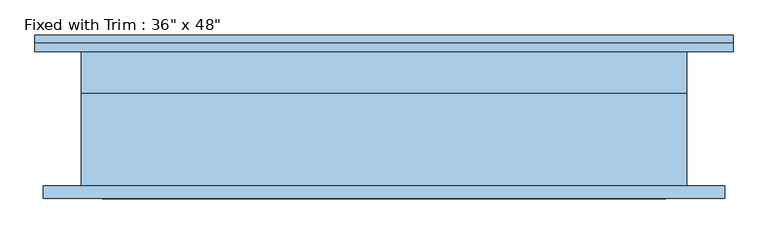
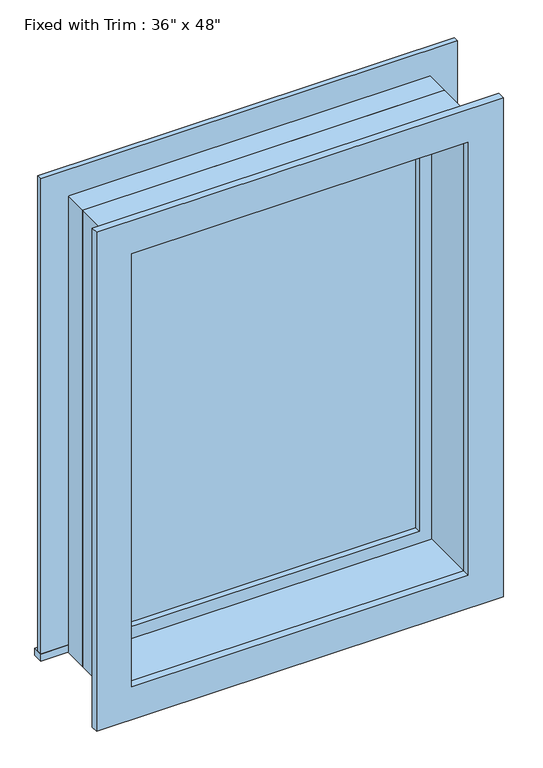
"""IFC4 building model written with IfcOpenShell, lengths in millimetres: window geometry."""

from ifc_helpers import new_model, si_unit, frame, origin, place, context, project, spatial, polyline, outline, extrude, source, transform, mapped, element, save


def window_bec2521a(model_context):
    return source(origin(), model_context, "Body", "SweptSolid", [
        extrude(outline(polyline([(-565.15, 127.0), (488.95, 127.0), (488.95, 101.6), (-565.15, 101.6), (-565.15, 127.0)])), frame((0.0, 0.0, 914.4), z_axis=(0.0, 0.0, 1.0), x_axis=(1.0, 0.0, 0.0)), (0.0, 0.0, 1.0), 19.05),
        extrude(outline(polyline([(2114.55, -476.25), (2114.55, 400.05), (933.45, 400.05), (933.45, 488.95), (2203.45, 488.95), (2203.45, -565.15), (933.45, -565.15), (933.45, -476.25), (2114.55, -476.25)])), frame((0.0, 101.6, 0.0), z_axis=(0.0, 1.0, 0.0), x_axis=(0.0, 0.0, 1.0)), (0.0, 0.0, 1.0), 12.7),
        extrude(outline(polyline([(2190.75, 476.25), (2190.75, -552.45), (857.25, -552.45), (857.25, 476.25), (2190.75, 476.25)]), holes=[polyline([(2101.85, 387.35), (946.15, 387.35), (946.15, -463.55), (2101.85, -463.55), (2101.85, 387.35)])]), frame((0.0, -120.65, 0.0), z_axis=(0.0, 1.0, 0.0), x_axis=(0.0, 0.0, 1.0)), (0.0, 0.0, 1.0), 19.05),
        extrude(outline(polyline([(355.6, 53.975), (-431.8, 53.975), (-431.8, 66.675), (355.6, 66.675), (355.6, 53.975)])), frame((0.0, 0.0, 977.9), z_axis=(0.0, 0.0, 1.0), x_axis=(1.0, 0.0, 0.0)), (0.0, 0.0, 1.0), 1092.2),
        extrude(outline(polyline([(2114.55, -476.25), (933.45, -476.25), (933.45, 400.05), (2114.55, 400.05), (2114.55, -476.25)]), holes=[polyline([(2070.1, -431.8), (2070.1, 355.6), (977.9, 355.6), (977.9, -431.8), (2070.1, -431.8)])]), frame((0.0, 38.1, 0.0), z_axis=(0.0, 1.0, 0.0), x_axis=(0.0, 0.0, 1.0)), (0.0, 0.0, 1.0), 44.45),
        extrude(outline(polyline([(2133.6, -495.3), (914.4, -495.3), (914.4, 419.1), (2133.6, 419.1), (2133.6, -495.3)]), holes=[polyline([(2101.85, -463.55), (2101.85, 387.35), (946.15, 387.35), (946.15, -463.55), (2101.85, -463.55)])]), frame((0.0, -101.6, 0.0), z_axis=(0.0, 1.0, 0.0), x_axis=(0.0, 0.0, 1.0)), (0.0, 0.0, 1.0), 139.7),
        extrude(outline(polyline([(2133.6, 419.1), (2133.6, -495.3), (914.4, -495.3), (914.4, 419.1), (2133.6, 419.1)]), holes=[polyline([(2114.55, 400.05), (933.45, 400.05), (933.45, -476.25), (2114.55, -476.25), (2114.55, 400.05)])]), frame((0.0, 38.1, 0.0), z_axis=(0.0, 1.0, 0.0), x_axis=(0.0, 0.0, 1.0)), (0.0, 0.0, 1.0), 63.5),
    ])


if __name__ == "__main__":
    model = new_model("IFC4")
    model_context = context("Model", 3, world=origin())
    ifc_project = project(units=[si_unit("LENGTHUNIT", "METRE", prefix="MILLI")], contexts=[model_context])
    site = spatial("IfcSite", under=ifc_project)
    building = spatial("IfcBuilding", under=site)
    placement = place(None, origin())
    window_shape = window_bec2521a(model_context)
    element("IfcWindow", 1, ObjectType="Fixed with Trim : 36\" x 48\"", at=placement, inside=building, context=model_context, shape_type="MappedRepresentation", body=[
        mapped(window_shape, transform((0.0, 0.0, 0.0), x_axis=(1.0, 0.0, 0.0), y_axis=(0.0, 1.0, 0.0), z_axis=(0.0, 0.0, 1.0))),
    ])
    save(model, "model.ifc")

# Revit data of these elements
# Type "Fixed with Trim : 36\" x 48\""
#   Type Mark = "13"
#   Construction Type Id = "GSP4R"
#   Assembly Code = "B2020100"
#   Analytic Construction = "1/8 in Pilkington single glazing"
#   Visual Light Transmittance = 0.9
#   Solar Heat Gain Coefficient = 0.78
#   Heat Transfer Coefficient (U) = 0.6496 BTU/(h·ft²·°F)
#   Height = 4' - 0"
#   Default Sill Height = 3' - 0"
#   Trim Projection - Ext. = 0' - 0 1/2"
#   Trim Projection - Int. = 0' - 0 3/4"
#   Trim Width - Exterior = 0' - 3 1/2"
#   Trim Width - Interior = 0' - 3 1/2"
#   Width = 3' - 0"
#   Window Inset = 0' - 0 3/4"
#   Define Thermal Properties by = 1
#   Glass Pane Material = Glass
#   Sash Material = Sash
#   Trim Exterior Material = Trim
#   Trim Interior Material = Trim
#   Wall Closure = (empty or 0)
# Element 1 (IfcWindow, "Fixed with Trim : 36\" x 48\"")
#   Materials on its faces: "Sash", "Trim", "Glass"
# Materials
#   "Glass": class "Glass", colour RGB 0 128 192, transparency 0.75, Description = "Soda Lime Glass", Cost = 0
#   "Sash": class "Wood", colour RGB 224 178 126, transparency 0
#   "Trim": class "Wood", colour RGB 224 178 126, transparency 0
